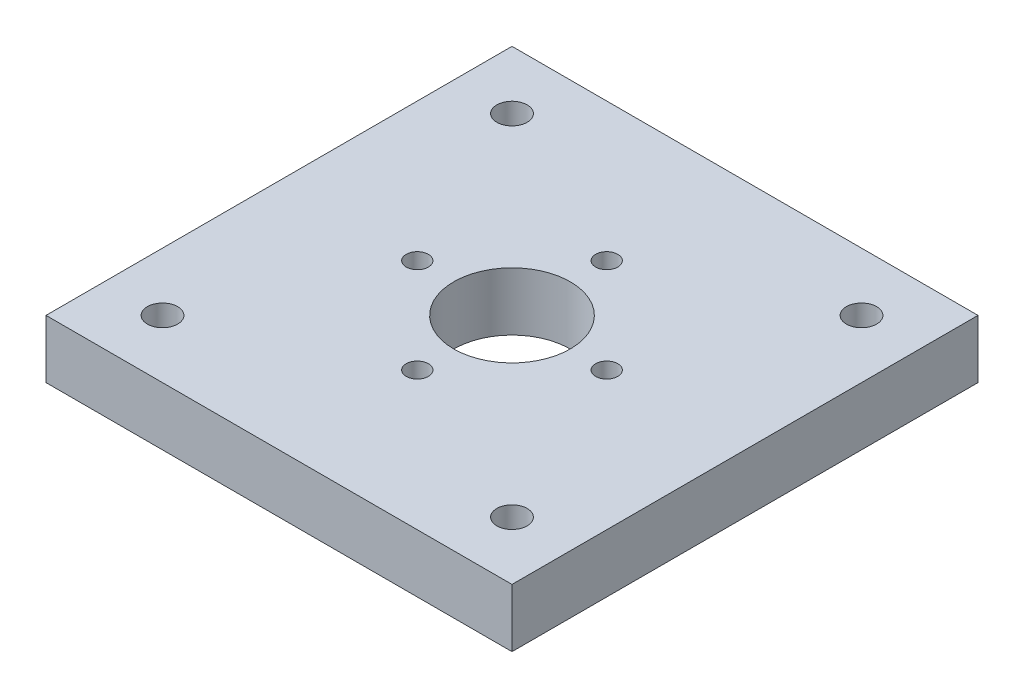
ISO-10303-21;
HEADER;
FILE_DESCRIPTION(('STEP AP214'),'2;1');
FILE_NAME('part.step','',(''),(''),'','','');
FILE_SCHEMA(('AUTOMOTIVE_DESIGN { 1 0 10303 214 1 1 1 1 }'));
ENDSEC;
DATA;
#1=APPLICATION_CONTEXT('core data for automotive mechanical design processes');
#2=APPLICATION_PROTOCOL_DEFINITION('international standard','automotive_design',2000,#1);
#3=PRODUCT_CONTEXT('',#1,'mechanical');
#4=PRODUCT('Part','Part','',(#3));
#5=PRODUCT_RELATED_PRODUCT_CATEGORY('part','',(#4));
#6=PRODUCT_DEFINITION_FORMATION('','',#4);
#7=PRODUCT_DEFINITION_CONTEXT('part definition',#1,'design');
#8=PRODUCT_DEFINITION('design','',#6,#7);
#9=PRODUCT_DEFINITION_SHAPE('','',#8);
#10=(LENGTH_UNIT() NAMED_UNIT(*) SI_UNIT(.MILLI.,.METRE.));
#11=(NAMED_UNIT(*) PLANE_ANGLE_UNIT() SI_UNIT($,.RADIAN.));
#12=(NAMED_UNIT(*) SI_UNIT($,.STERADIAN.) SOLID_ANGLE_UNIT());
#13=UNCERTAINTY_MEASURE_WITH_UNIT(LENGTH_MEASURE(1.E-05),#10,'distance_accuracy_value','');
#14=(GEOMETRIC_REPRESENTATION_CONTEXT(3) GLOBAL_UNCERTAINTY_ASSIGNED_CONTEXT((#13)) GLOBAL_UNIT_ASSIGNED_CONTEXT((#10,
#11,#12)) REPRESENTATION_CONTEXT('',''));
#15=CARTESIAN_POINT('',(0.,0.,0.));
#16=DIRECTION('',(0.,0.,1.));
#17=DIRECTION('',(1.,0.,0.));
#18=AXIS2_PLACEMENT_3D('',#15,#16,#17);
#19=CARTESIAN_POINT('',(0.,25.,0.));
#20=DIRECTION('',(0.,-1.,0.));
#21=DIRECTION('',(0.,0.,-1.));
#22=AXIS2_PLACEMENT_3D('',#19,#20,#21);
#23=PLANE('',#22);
#24=DIRECTION('',(0.,0.,-1.));
#25=VECTOR('',#24,1.);
#26=CARTESIAN_POINT('',(200.,25.,200.));
#27=LINE('',#26,#25);
#28=CARTESIAN_POINT('',(200.,25.,200.));
#29=VERTEX_POINT('',#28);
#30=CARTESIAN_POINT('',(200.,25.,-200.));
#31=VERTEX_POINT('',#30);
#32=EDGE_CURVE('E93',#29,#31,#27,.T.);
#33=ORIENTED_EDGE('',*,*,#32,.T.);
#34=DIRECTION('',(-1.,0.,0.));
#35=VECTOR('',#34,1.);
#36=CARTESIAN_POINT('',(-200.,25.,-200.));
#37=LINE('',#36,#35);
#38=CARTESIAN_POINT('',(-200.,25.,-200.));
#39=VERTEX_POINT('',#38);
#40=EDGE_CURVE('E88',#31,#39,#37,.T.);
#41=ORIENTED_EDGE('',*,*,#40,.T.);
#42=DIRECTION('',(0.,0.,1.));
#43=VECTOR('',#42,1.);
#44=CARTESIAN_POINT('',(-200.,25.,200.));
#45=LINE('',#44,#43);
#46=CARTESIAN_POINT('',(-200.,25.,200.));
#47=VERTEX_POINT('',#46);
#48=EDGE_CURVE('E90',#39,#47,#45,.T.);
#49=ORIENTED_EDGE('',*,*,#48,.T.);
#50=DIRECTION('',(1.,0.,0.));
#51=VECTOR('',#50,1.);
#52=CARTESIAN_POINT('',(-200.,25.,200.));
#53=LINE('',#52,#51);
#54=EDGE_CURVE('E57',#47,#29,#53,.T.);
#55=ORIENTED_EDGE('',*,*,#54,.T.);
#56=EDGE_LOOP('',(#33,#41,#49,#55));
#57=FACE_BOUND('',#56,.T.);
#58=CARTESIAN_POINT('',(-1.11022302462516E-13,25.,0.));
#59=DIRECTION('',(0.,1.,0.));
#60=DIRECTION('',(0.,0.,1.));
#61=AXIS2_PLACEMENT_3D('',#58,#59,#60);
#62=CIRCLE('',#61,50.);
#63=CARTESIAN_POINT('',(-1.11022302462516E-13,25.,50.0000000000001));
#64=VERTEX_POINT('',#63);
#65=EDGE_CURVE('E106',#64,#64,#62,.T.);
#66=ORIENTED_EDGE('',*,*,#65,.F.);
#67=EDGE_LOOP('',(#66));
#68=FACE_BOUND('',#67,.T.);
#69=CARTESIAN_POINT('',(150.,25.,-150.));
#70=DIRECTION('',(0.,1.,0.));
#71=DIRECTION('',(0.,0.,1.));
#72=AXIS2_PLACEMENT_3D('',#69,#70,#71);
#73=CIRCLE('',#72,13.);
#74=CARTESIAN_POINT('',(150.,25.,-137.));
#75=VERTEX_POINT('',#74);
#76=EDGE_CURVE('E122',#75,#75,#73,.T.);
#77=ORIENTED_EDGE('',*,*,#76,.F.);
#78=EDGE_LOOP('',(#77));
#79=FACE_BOUND('',#78,.T.);
#80=CARTESIAN_POINT('',(-150.,25.,-150.));
#81=DIRECTION('',(0.,1.,0.));
#82=DIRECTION('',(0.,0.,-1.));
#83=AXIS2_PLACEMENT_3D('',#80,#81,#82);
#84=CIRCLE('',#83,13.);
#85=CARTESIAN_POINT('',(-150.,25.,-163.));
#86=VERTEX_POINT('',#85);
#87=EDGE_CURVE('E130',#86,#86,#84,.T.);
#88=ORIENTED_EDGE('',*,*,#87,.F.);
#89=EDGE_LOOP('',(#88));
#90=FACE_BOUND('',#89,.T.);
#91=CARTESIAN_POINT('',(150.,25.,150.));
#92=DIRECTION('',(0.,1.,0.));
#93=DIRECTION('',(0.,0.,-1.));
#94=AXIS2_PLACEMENT_3D('',#91,#92,#93);
#95=CIRCLE('',#94,13.);
#96=CARTESIAN_POINT('',(150.,25.,137.));
#97=VERTEX_POINT('',#96);
#98=EDGE_CURVE('E134',#97,#97,#95,.T.);
#99=ORIENTED_EDGE('',*,*,#98,.F.);
#100=EDGE_LOOP('',(#99));
#101=FACE_BOUND('',#100,.T.);
#102=CARTESIAN_POINT('',(-150.,25.,150.));
#103=DIRECTION('',(0.,1.,0.));
#104=DIRECTION('',(0.,0.,1.));
#105=AXIS2_PLACEMENT_3D('',#102,#103,#104);
#106=CIRCLE('',#105,13.);
#107=CARTESIAN_POINT('',(-150.,25.,163.));
#108=VERTEX_POINT('',#107);
#109=EDGE_CURVE('E136',#108,#108,#106,.T.);
#110=ORIENTED_EDGE('',*,*,#109,.F.);
#111=EDGE_LOOP('',(#110));
#112=FACE_BOUND('',#111,.T.);
#113=CARTESIAN_POINT('',(-1.11022302462516E-13,25.,-81.2999999999999));
#114=DIRECTION('',(0.,1.,0.));
#115=DIRECTION('',(0.,0.,1.));
#116=AXIS2_PLACEMENT_3D('',#113,#114,#115);
#117=CIRCLE('',#116,9.5);
#118=CARTESIAN_POINT('',(-1.11022302462516E-13,25.,-71.7999999999999));
#119=VERTEX_POINT('',#118);
#120=EDGE_CURVE('E144',#119,#119,#117,.T.);
#121=ORIENTED_EDGE('',*,*,#120,.F.);
#122=EDGE_LOOP('',(#121));
#123=FACE_BOUND('',#122,.T.);
#124=CARTESIAN_POINT('',(-1.11022302462516E-13,25.,81.3));
#125=DIRECTION('',(0.,1.,0.));
#126=DIRECTION('',(0.,0.,-1.));
#127=AXIS2_PLACEMENT_3D('',#124,#125,#126);
#128=CIRCLE('',#127,9.5);
#129=CARTESIAN_POINT('',(-1.11022302462516E-13,25.,71.8));
#130=VERTEX_POINT('',#129);
#131=EDGE_CURVE('E151',#130,#130,#128,.T.);
#132=ORIENTED_EDGE('',*,*,#131,.F.);
#133=EDGE_LOOP('',(#132));
#134=FACE_BOUND('',#133,.T.);
#135=CARTESIAN_POINT('',(-81.3000000000001,25.,0.));
#136=DIRECTION('',(0.,1.,0.));
#137=DIRECTION('',(0.,0.,1.));
#138=AXIS2_PLACEMENT_3D('',#135,#136,#137);
#139=CIRCLE('',#138,9.49999999999999);
#140=CARTESIAN_POINT('',(-81.3000000000001,25.,9.50000000000005));
#141=VERTEX_POINT('',#140);
#142=EDGE_CURVE('E160',#141,#141,#139,.T.);
#143=ORIENTED_EDGE('',*,*,#142,.F.);
#144=EDGE_LOOP('',(#143));
#145=FACE_BOUND('',#144,.T.);
#146=CARTESIAN_POINT('',(81.3,25.,0.));
#147=DIRECTION('',(0.,1.,0.));
#148=DIRECTION('',(0.,0.,-1.));
#149=AXIS2_PLACEMENT_3D('',#146,#147,#148);
#150=CIRCLE('',#149,9.49999999999999);
#151=CARTESIAN_POINT('',(81.3,25.,-9.49999999999994));
#152=VERTEX_POINT('',#151);
#153=EDGE_CURVE('E162',#152,#152,#150,.T.);
#154=ORIENTED_EDGE('',*,*,#153,.F.);
#155=EDGE_LOOP('',(#154));
#156=FACE_BOUND('',#155,.T.);
#157=ADVANCED_FACE('F39',(#57,#68,#79,#90,#101,#112,#123,#134,#145,#156),#23,.F.);
#158=CARTESIAN_POINT('',(0.,-25.,0.));
#159=DIRECTION('',(0.,-1.,0.));
#160=DIRECTION('',(0.,0.,-1.));
#161=AXIS2_PLACEMENT_3D('',#158,#159,#160);
#162=PLANE('',#161);
#163=CARTESIAN_POINT('',(-81.3000000000001,-25.,0.));
#164=DIRECTION('',(0.,1.,0.));
#165=DIRECTION('',(0.,0.,1.));
#166=AXIS2_PLACEMENT_3D('',#163,#164,#165);
#167=CIRCLE('',#166,9.49999999999999);
#168=CARTESIAN_POINT('',(-81.3000000000001,-25.,9.50000000000005));
#169=VERTEX_POINT('',#168);
#170=EDGE_CURVE('E159',#169,#169,#167,.T.);
#171=ORIENTED_EDGE('',*,*,#170,.T.);
#172=EDGE_LOOP('',(#171));
#173=FACE_BOUND('',#172,.T.);
#174=CARTESIAN_POINT('',(-1.11022302462516E-13,-25.,-81.2999999999999));
#175=DIRECTION('',(0.,1.,0.));
#176=DIRECTION('',(0.,0.,1.));
#177=AXIS2_PLACEMENT_3D('',#174,#175,#176);
#178=CIRCLE('',#177,9.5);
#179=CARTESIAN_POINT('',(-1.11022302462516E-13,-25.,-71.7999999999999));
#180=VERTEX_POINT('',#179);
#181=EDGE_CURVE('E146',#180,#180,#178,.T.);
#182=ORIENTED_EDGE('',*,*,#181,.T.);
#183=EDGE_LOOP('',(#182));
#184=FACE_BOUND('',#183,.T.);
#185=CARTESIAN_POINT('',(150.,-25.,150.));
#186=DIRECTION('',(0.,1.,0.));
#187=DIRECTION('',(0.,0.,-1.));
#188=AXIS2_PLACEMENT_3D('',#185,#186,#187);
#189=CIRCLE('',#188,13.);
#190=CARTESIAN_POINT('',(150.,-25.,137.));
#191=VERTEX_POINT('',#190);
#192=EDGE_CURVE('E137',#191,#191,#189,.T.);
#193=ORIENTED_EDGE('',*,*,#192,.T.);
#194=EDGE_LOOP('',(#193));
#195=FACE_BOUND('',#194,.T.);
#196=CARTESIAN_POINT('',(150.,-25.,-150.));
#197=DIRECTION('',(0.,1.,0.));
#198=DIRECTION('',(0.,0.,1.));
#199=AXIS2_PLACEMENT_3D('',#196,#197,#198);
#200=CIRCLE('',#199,13.);
#201=CARTESIAN_POINT('',(150.,-25.,-137.));
#202=VERTEX_POINT('',#201);
#203=EDGE_CURVE('E121',#202,#202,#200,.T.);
#204=ORIENTED_EDGE('',*,*,#203,.T.);
#205=EDGE_LOOP('',(#204));
#206=FACE_BOUND('',#205,.T.);
#207=DIRECTION('',(0.,0.,-1.));
#208=VECTOR('',#207,1.);
#209=CARTESIAN_POINT('',(200.,-25.,200.));
#210=LINE('',#209,#208);
#211=CARTESIAN_POINT('',(200.,-25.,200.));
#212=VERTEX_POINT('',#211);
#213=CARTESIAN_POINT('',(200.,-25.,-200.));
#214=VERTEX_POINT('',#213);
#215=EDGE_CURVE('E103',#212,#214,#210,.T.);
#216=ORIENTED_EDGE('',*,*,#215,.F.);
#217=DIRECTION('',(1.,0.,0.));
#218=VECTOR('',#217,1.);
#219=CARTESIAN_POINT('',(-200.,-25.,200.));
#220=LINE('',#219,#218);
#221=CARTESIAN_POINT('',(-200.,-25.,200.));
#222=VERTEX_POINT('',#221);
#223=EDGE_CURVE('E76',#222,#212,#220,.T.);
#224=ORIENTED_EDGE('',*,*,#223,.F.);
#225=DIRECTION('',(0.,0.,1.));
#226=VECTOR('',#225,1.);
#227=CARTESIAN_POINT('',(-200.,-25.,200.));
#228=LINE('',#227,#226);
#229=CARTESIAN_POINT('',(-200.,-25.,-200.));
#230=VERTEX_POINT('',#229);
#231=EDGE_CURVE('E71',#230,#222,#228,.T.);
#232=ORIENTED_EDGE('',*,*,#231,.F.);
#233=DIRECTION('',(-1.,0.,0.));
#234=VECTOR('',#233,1.);
#235=CARTESIAN_POINT('',(-200.,-25.,-200.));
#236=LINE('',#235,#234);
#237=EDGE_CURVE('E92',#214,#230,#236,.T.);
#238=ORIENTED_EDGE('',*,*,#237,.F.);
#239=EDGE_LOOP('',(#216,#224,#232,#238));
#240=FACE_BOUND('',#239,.T.);
#241=CARTESIAN_POINT('',(-1.11022302462516E-13,-25.,0.));
#242=DIRECTION('',(0.,1.,0.));
#243=DIRECTION('',(0.,0.,1.));
#244=AXIS2_PLACEMENT_3D('',#241,#242,#243);
#245=CIRCLE('',#244,50.);
#246=CARTESIAN_POINT('',(-1.11022302462516E-13,-25.,50.0000000000001));
#247=VERTEX_POINT('',#246);
#248=EDGE_CURVE('E119',#247,#247,#245,.T.);
#249=ORIENTED_EDGE('',*,*,#248,.T.);
#250=EDGE_LOOP('',(#249));
#251=FACE_BOUND('',#250,.T.);
#252=CARTESIAN_POINT('',(-150.,-25.,-150.));
#253=DIRECTION('',(0.,1.,0.));
#254=DIRECTION('',(0.,0.,-1.));
#255=AXIS2_PLACEMENT_3D('',#252,#253,#254);
#256=CIRCLE('',#255,13.);
#257=CARTESIAN_POINT('',(-150.,-25.,-163.));
#258=VERTEX_POINT('',#257);
#259=EDGE_CURVE('E128',#258,#258,#256,.T.);
#260=ORIENTED_EDGE('',*,*,#259,.T.);
#261=EDGE_LOOP('',(#260));
#262=FACE_BOUND('',#261,.T.);
#263=CARTESIAN_POINT('',(-150.,-25.,150.));
#264=DIRECTION('',(0.,1.,0.));
#265=DIRECTION('',(0.,0.,1.));
#266=AXIS2_PLACEMENT_3D('',#263,#264,#265);
#267=CIRCLE('',#266,13.);
#268=CARTESIAN_POINT('',(-150.,-25.,163.));
#269=VERTEX_POINT('',#268);
#270=EDGE_CURVE('E142',#269,#269,#267,.T.);
#271=ORIENTED_EDGE('',*,*,#270,.T.);
#272=EDGE_LOOP('',(#271));
#273=FACE_BOUND('',#272,.T.);
#274=CARTESIAN_POINT('',(-1.11022302462516E-13,-25.,81.3));
#275=DIRECTION('',(0.,1.,0.));
#276=DIRECTION('',(0.,0.,-1.));
#277=AXIS2_PLACEMENT_3D('',#274,#275,#276);
#278=CIRCLE('',#277,9.5);
#279=CARTESIAN_POINT('',(-1.11022302462516E-13,-25.,71.8));
#280=VERTEX_POINT('',#279);
#281=EDGE_CURVE('E152',#280,#280,#278,.T.);
#282=ORIENTED_EDGE('',*,*,#281,.T.);
#283=EDGE_LOOP('',(#282));
#284=FACE_BOUND('',#283,.T.);
#285=CARTESIAN_POINT('',(81.3,-25.,0.));
#286=DIRECTION('',(0.,1.,0.));
#287=DIRECTION('',(0.,0.,-1.));
#288=AXIS2_PLACEMENT_3D('',#285,#286,#287);
#289=CIRCLE('',#288,9.49999999999999);
#290=CARTESIAN_POINT('',(81.3,-25.,-9.49999999999994));
#291=VERTEX_POINT('',#290);
#292=EDGE_CURVE('E167',#291,#291,#289,.T.);
#293=ORIENTED_EDGE('',*,*,#292,.T.);
#294=EDGE_LOOP('',(#293));
#295=FACE_BOUND('',#294,.T.);
#296=ADVANCED_FACE('F111',(#173,#184,#195,#206,#240,#251,#262,#273,#284,#295),#162,.T.);
#297=CARTESIAN_POINT('',(200.,25.,200.));
#298=DIRECTION('',(-1.,0.,0.));
#299=DIRECTION('',(0.,0.,1.));
#300=AXIS2_PLACEMENT_3D('',#297,#298,#299);
#301=PLANE('',#300);
#302=ORIENTED_EDGE('',*,*,#215,.T.);
#303=DIRECTION('',(0.,-1.,0.));
#304=VECTOR('',#303,1.);
#305=CARTESIAN_POINT('',(200.,25.,-200.));
#306=LINE('',#305,#304);
#307=EDGE_CURVE('E11',#31,#214,#306,.T.);
#308=ORIENTED_EDGE('',*,*,#307,.F.);
#309=ORIENTED_EDGE('',*,*,#32,.F.);
#310=DIRECTION('',(0.,-1.,0.));
#311=VECTOR('',#310,1.);
#312=CARTESIAN_POINT('',(200.,25.,200.));
#313=LINE('',#312,#311);
#314=EDGE_CURVE('E97',#29,#212,#313,.T.);
#315=ORIENTED_EDGE('',*,*,#314,.T.);
#316=EDGE_LOOP('',(#302,#308,#309,#315));
#317=FACE_BOUND('',#316,.T.);
#318=ADVANCED_FACE('F41',(#317),#301,.F.);
#319=CARTESIAN_POINT('',(-200.,25.,-200.));
#320=DIRECTION('',(0.,0.,1.));
#321=DIRECTION('',(1.,0.,0.));
#322=AXIS2_PLACEMENT_3D('',#319,#320,#321);
#323=PLANE('',#322);
#324=ORIENTED_EDGE('',*,*,#237,.T.);
#325=DIRECTION('',(0.,-1.,0.));
#326=VECTOR('',#325,1.);
#327=CARTESIAN_POINT('',(-200.,25.,-200.));
#328=LINE('',#327,#326);
#329=EDGE_CURVE('E48',#39,#230,#328,.T.);
#330=ORIENTED_EDGE('',*,*,#329,.F.);
#331=ORIENTED_EDGE('',*,*,#40,.F.);
#332=ORIENTED_EDGE('',*,*,#307,.T.);
#333=EDGE_LOOP('',(#324,#330,#331,#332));
#334=FACE_BOUND('',#333,.T.);
#335=ADVANCED_FACE('F94',(#334),#323,.F.);
#336=CARTESIAN_POINT('',(-200.,25.,200.));
#337=DIRECTION('',(1.,0.,0.));
#338=DIRECTION('',(0.,0.,-1.));
#339=AXIS2_PLACEMENT_3D('',#336,#337,#338);
#340=PLANE('',#339);
#341=ORIENTED_EDGE('',*,*,#231,.T.);
#342=DIRECTION('',(0.,-1.,0.));
#343=VECTOR('',#342,1.);
#344=CARTESIAN_POINT('',(-200.,25.,200.));
#345=LINE('',#344,#343);
#346=EDGE_CURVE('E96',#47,#222,#345,.T.);
#347=ORIENTED_EDGE('',*,*,#346,.F.);
#348=ORIENTED_EDGE('',*,*,#48,.F.);
#349=ORIENTED_EDGE('',*,*,#329,.T.);
#350=EDGE_LOOP('',(#341,#347,#348,#349));
#351=FACE_BOUND('',#350,.T.);
#352=ADVANCED_FACE('F100',(#351),#340,.F.);
#353=CARTESIAN_POINT('',(-200.,25.,200.));
#354=DIRECTION('',(0.,0.,-1.));
#355=DIRECTION('',(-1.,0.,0.));
#356=AXIS2_PLACEMENT_3D('',#353,#354,#355);
#357=PLANE('',#356);
#358=ORIENTED_EDGE('',*,*,#223,.T.);
#359=ORIENTED_EDGE('',*,*,#314,.F.);
#360=ORIENTED_EDGE('',*,*,#54,.F.);
#361=ORIENTED_EDGE('',*,*,#346,.T.);
#362=EDGE_LOOP('',(#358,#359,#360,#361));
#363=FACE_BOUND('',#362,.T.);
#364=ADVANCED_FACE('F112',(#363),#357,.F.);
#365=CARTESIAN_POINT('',(-1.11022302462516E-13,25.,0.));
#366=DIRECTION('',(0.,-1.,0.));
#367=DIRECTION('',(0.,0.,-1.));
#368=AXIS2_PLACEMENT_3D('',#365,#366,#367);
#369=CYLINDRICAL_SURFACE('',#368,50.);
#370=ORIENTED_EDGE('',*,*,#65,.T.);
#371=EDGE_LOOP('',(#370));
#372=FACE_BOUND('',#371,.T.);
#373=ORIENTED_EDGE('',*,*,#248,.F.);
#374=EDGE_LOOP('',(#373));
#375=FACE_BOUND('',#374,.T.);
#376=ADVANCED_FACE('F181',(#372,#375),#369,.F.);
#377=CARTESIAN_POINT('',(150.,25.,-150.));
#378=DIRECTION('',(0.,-1.,0.));
#379=DIRECTION('',(0.,0.,-1.));
#380=AXIS2_PLACEMENT_3D('',#377,#378,#379);
#381=CYLINDRICAL_SURFACE('',#380,13.);
#382=ORIENTED_EDGE('',*,*,#76,.T.);
#383=EDGE_LOOP('',(#382));
#384=FACE_BOUND('',#383,.T.);
#385=ORIENTED_EDGE('',*,*,#203,.F.);
#386=EDGE_LOOP('',(#385));
#387=FACE_BOUND('',#386,.T.);
#388=ADVANCED_FACE('F229',(#384,#387),#381,.F.);
#389=CARTESIAN_POINT('',(-150.,25.,-150.));
#390=DIRECTION('',(0.,-1.,0.));
#391=DIRECTION('',(0.,0.,-1.));
#392=AXIS2_PLACEMENT_3D('',#389,#390,#391);
#393=CYLINDRICAL_SURFACE('',#392,13.);
#394=ORIENTED_EDGE('',*,*,#87,.T.);
#395=EDGE_LOOP('',(#394));
#396=FACE_BOUND('',#395,.T.);
#397=ORIENTED_EDGE('',*,*,#259,.F.);
#398=EDGE_LOOP('',(#397));
#399=FACE_BOUND('',#398,.T.);
#400=ADVANCED_FACE('F237',(#396,#399),#393,.F.);
#401=CARTESIAN_POINT('',(150.,25.,150.));
#402=DIRECTION('',(0.,-1.,0.));
#403=DIRECTION('',(0.,0.,-1.));
#404=AXIS2_PLACEMENT_3D('',#401,#402,#403);
#405=CYLINDRICAL_SURFACE('',#404,13.);
#406=ORIENTED_EDGE('',*,*,#98,.T.);
#407=EDGE_LOOP('',(#406));
#408=FACE_BOUND('',#407,.T.);
#409=ORIENTED_EDGE('',*,*,#192,.F.);
#410=EDGE_LOOP('',(#409));
#411=FACE_BOUND('',#410,.T.);
#412=ADVANCED_FACE('F241',(#408,#411),#405,.F.);
#413=CARTESIAN_POINT('',(-150.,25.,150.));
#414=DIRECTION('',(0.,-1.,0.));
#415=DIRECTION('',(0.,0.,-1.));
#416=AXIS2_PLACEMENT_3D('',#413,#414,#415);
#417=CYLINDRICAL_SURFACE('',#416,13.);
#418=ORIENTED_EDGE('',*,*,#109,.T.);
#419=EDGE_LOOP('',(#418));
#420=FACE_BOUND('',#419,.T.);
#421=ORIENTED_EDGE('',*,*,#270,.F.);
#422=EDGE_LOOP('',(#421));
#423=FACE_BOUND('',#422,.T.);
#424=ADVANCED_FACE('F251',(#420,#423),#417,.F.);
#425=CARTESIAN_POINT('',(-1.11022302462516E-13,25.,-81.2999999999999));
#426=DIRECTION('',(0.,-1.,0.));
#427=DIRECTION('',(0.,0.,-1.));
#428=AXIS2_PLACEMENT_3D('',#425,#426,#427);
#429=CYLINDRICAL_SURFACE('',#428,9.5);
#430=ORIENTED_EDGE('',*,*,#120,.T.);
#431=EDGE_LOOP('',(#430));
#432=FACE_BOUND('',#431,.T.);
#433=ORIENTED_EDGE('',*,*,#181,.F.);
#434=EDGE_LOOP('',(#433));
#435=FACE_BOUND('',#434,.T.);
#436=ADVANCED_FACE('F265',(#432,#435),#429,.F.);
#437=CARTESIAN_POINT('',(-1.11022302462516E-13,25.,81.3));
#438=DIRECTION('',(0.,-1.,0.));
#439=DIRECTION('',(0.,0.,-1.));
#440=AXIS2_PLACEMENT_3D('',#437,#438,#439);
#441=CYLINDRICAL_SURFACE('',#440,9.5);
#442=ORIENTED_EDGE('',*,*,#131,.T.);
#443=EDGE_LOOP('',(#442));
#444=FACE_BOUND('',#443,.T.);
#445=ORIENTED_EDGE('',*,*,#281,.F.);
#446=EDGE_LOOP('',(#445));
#447=FACE_BOUND('',#446,.T.);
#448=ADVANCED_FACE('F271',(#444,#447),#441,.F.);
#449=CARTESIAN_POINT('',(-81.3000000000001,25.,0.));
#450=DIRECTION('',(0.,-1.,0.));
#451=DIRECTION('',(0.,0.,-1.));
#452=AXIS2_PLACEMENT_3D('',#449,#450,#451);
#453=CYLINDRICAL_SURFACE('',#452,9.49999999999999);
#454=ORIENTED_EDGE('',*,*,#142,.T.);
#455=EDGE_LOOP('',(#454));
#456=FACE_BOUND('',#455,.T.);
#457=ORIENTED_EDGE('',*,*,#170,.F.);
#458=EDGE_LOOP('',(#457));
#459=FACE_BOUND('',#458,.T.);
#460=ADVANCED_FACE('F278',(#456,#459),#453,.F.);
#461=CARTESIAN_POINT('',(81.3,25.,0.));
#462=DIRECTION('',(0.,-1.,0.));
#463=DIRECTION('',(0.,0.,-1.));
#464=AXIS2_PLACEMENT_3D('',#461,#462,#463);
#465=CYLINDRICAL_SURFACE('',#464,9.49999999999999);
#466=ORIENTED_EDGE('',*,*,#153,.T.);
#467=EDGE_LOOP('',(#466));
#468=FACE_BOUND('',#467,.T.);
#469=ORIENTED_EDGE('',*,*,#292,.F.);
#470=EDGE_LOOP('',(#469));
#471=FACE_BOUND('',#470,.T.);
#472=ADVANCED_FACE('F175',(#468,#471),#465,.F.);
#473=CLOSED_SHELL('',(#157,#296,#318,#335,#352,#364,#376,#388,#400,#412,#424,#436,#448,#460,#472));
#474=MANIFOLD_SOLID_BREP('B2',#473);
#475=ADVANCED_BREP_SHAPE_REPRESENTATION('',(#18,#474),#14);
#476=SHAPE_DEFINITION_REPRESENTATION(#9,#475);
ENDSEC;
END-ISO-10303-21;
